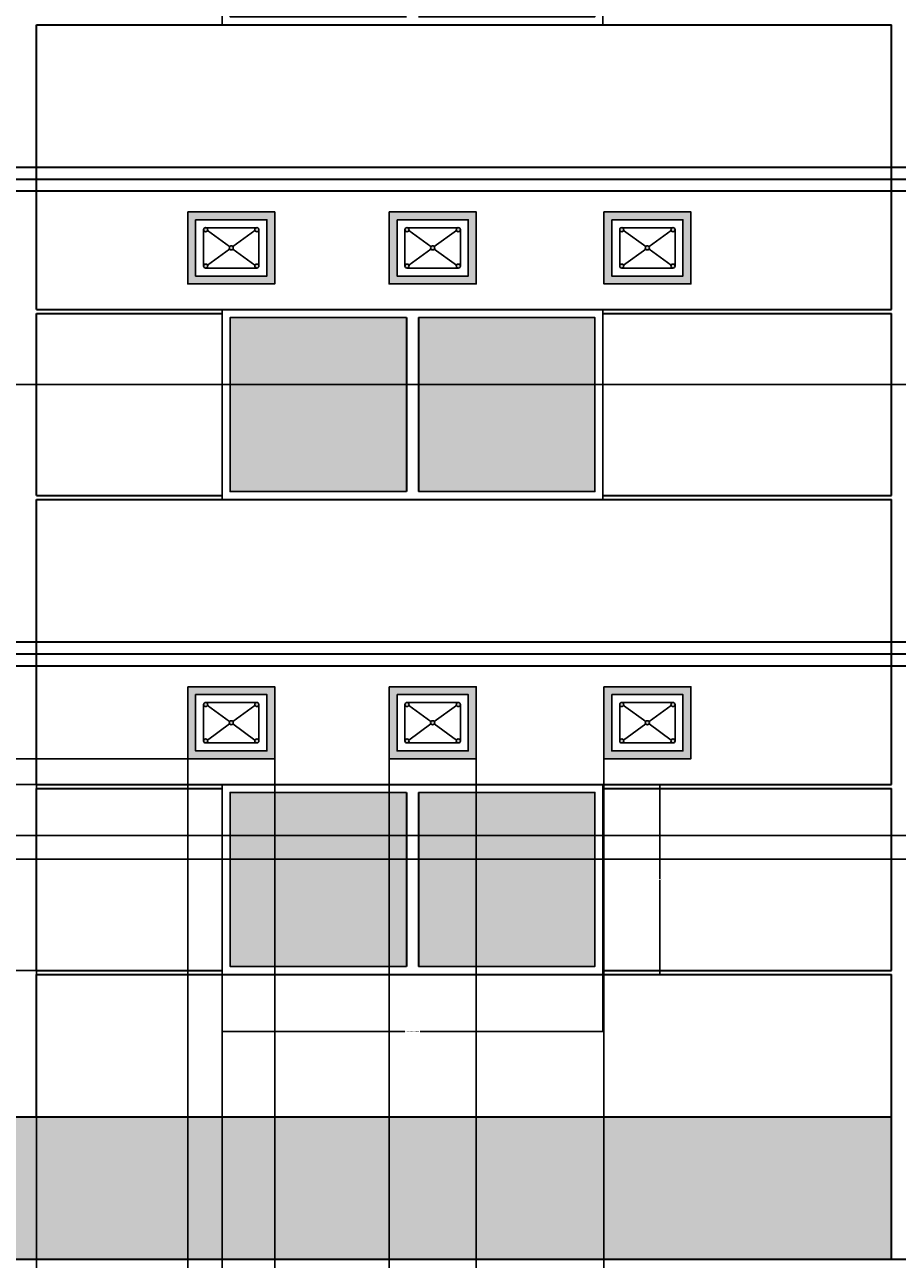
# Model space of a CAD drawing. Units: inches. Extents: x -742 to 1386, y -64 to 951.
# Tile 4 of 8: x 43 to 264, y 106 to 418. Entities that reach past the tile are written whole.
import ezdxf

# ---------------------------------------------------------------- set-up
doc = ezdxf.new("R2010")
doc.units = ezdxf.units.IN
doc.header["$MEASUREMENT"] = 0
for name, color, linetype, lineweight in [('A-ANNO-DIMS', 2, 'Continuous', 18), ('A-ELEV', 7, 'Continuous', 35), ('A-ELEV-PATT', 252, 'Continuous', 13), ('A-GLAZ', 4, 'Continuous', 25), ('A-WALL-PATT', 8, 'Continuous', 13)]:
    doc.layers.add(name, color=color, linetype=linetype, lineweight=lineweight)
doc.styles.get("Standard").update_dxf_attribs({"font": 'arial.ttf'})
doc.dimstyles.get("Standard").update_dxf_attribs({"dimtxt": 0.18, "dimasz": 0.18, "dimexe": 0.18, "dimexo": 0.0625, "dimgap": 0.09, "dimtad": 0, "dimtih": 1, "dimtoh": 1, "dimdec": 4, "dimzin": 0, "dimdsep": 46, "dimtxsty": 'Standard', "dimcen": 0.09, "dimadec": 0, "dimazin": 0, "dimtfac": 1, "dimtdec": 4, "dimtofl": 0, "dimtmove": 0, "dimatfit": 3, "dimfxl": 1, "dimtolj": 1, "dimtzin": 0, "dimarcsym": 0})

# ---------------------------------------------------------------- blocks, each defined once
blk = doc.blocks.new('VENT-WIN')
h = blk.add_hatch(color=256)
h.dxf.hatch_style = 1
h.paths.add_polyline_path([(11.51, 9.11, 1), (10.47, 9.11, 1)])
h.paths.add_polyline_path([(16.95, 13.71, 1), (17.99, 13.71, 1)])
h.paths.add_polyline_path([(17.99, 4.52, 1), (16.95, 4.52, 1)])
h.paths.add_polyline_path([(5.04, 4.52, 1), (4, 4.52, 1)])
h.paths.add_polyline_path([(4, 13.71, 1), (5.04, 13.71, 1)])
for p, q in [((4.99, 13.5), (10.57, 9.42)), ((11.41, 9.42), (16.99, 13.5)), ((4.99, 4.73), (10.57, 8.81)), ((11.41, 8.81), (16.99, 4.73))]:
    blk.add_line(p, q)
for points in [[(0, 18.22), (21.99, 18.22), (21.99, 0), (0, 0)], [(2, 16.22), (19.99, 16.22), (19.99, 2), (2, 2)]]:
    blk.add_lwpolyline(points, close=True)
for points in [[(4, 4.52), (4, 13.71)], [(4.52, 14.22), (17.47, 14.22)], [(17.99, 13.71), (17.99, 4.52)], [(17.47, 4), (4.52, 4)]]:
    blk.add_lwpolyline(points)
for centre in [(4.52, 13.71), (17.47, 13.71), (10.99, 9.11), (4.52, 4.52), (17.47, 4.52)]:
    blk.add_circle(centre, 0.519)
blk = doc.blocks.new('WIN-1000-2PANE')
blk.add_lwpolyline([(0, 48), (96.2, 48), (96.2, 0), (0, 0)], close=True)
for points in [[(46.6, 2), (2, 2), (2, 46), (46.6, 46)], [(49.6, 46), (94.2, 46), (94.2, 2), (49.6, 2)]]:
    blk.add_lwpolyline(points)
blk = doc.blocks.new('*D8')
at = {"layer": 'A-ANNO-DIMS', "color": 0, "lineweight": -2, "transparency": 16777216}
for p, q in [((93.11, 177.68), (93.11, 163.13)), ((189.31, 177.68), (189.31, 163.13)), ((93.29, 163.31), (139.29, 163.31)), ((189.13, 163.31), (143.13, 163.31))]:
    blk.add_line(p, q, dxfattribs=at)
at = {"layer": 'A-ANNO-DIMS', "color": 0, "transparency": 16777216}
for points in [[(93.29, 163.34), (93.29, 163.28), (93.11, 163.31)], [(189.13, 163.34), (189.13, 163.28), (189.31, 163.31)]]:
    blk.add_solid(points, dxfattribs=at)
at = {"layer": 'Defpoints', "color": 0, "transparency": 16777216}
for p in [(93.11, 177.74), (189.31, 177.74), (189.31, 163.31)]:
    blk.add_point(p, dxfattribs=at)
at = {"layer": 'A-ANNO-DIMS', "color": 0, "transparency": 16777216, "insert": (141.21, 163.31), "char_height": 0.18, "attachment_point": 5}
blk.add_mtext('\\A1;WINDOW 1000 2-PANE 96 TYP.', dxfattribs=at)
blk = doc.blocks.new('*D9')
at = {"layer": 'A-ANNO-DIMS', "color": 0, "lineweight": -2, "transparency": 16777216}
for p, q in [((189.38, 225.74), (203.92, 225.74)), ((203.74, 225.56), (203.74, 201.92)), ((203.74, 177.92), (203.74, 201.56)), ((189.38, 177.74), (203.92, 177.74))]:
    blk.add_line(p, q, dxfattribs=at)
at = {"layer": 'A-ANNO-DIMS', "color": 0, "transparency": 16777216}
for points in [[(203.71, 225.56), (203.77, 225.56), (203.74, 225.74)], [(203.71, 177.92), (203.77, 177.92), (203.74, 177.74)]]:
    blk.add_solid(points, dxfattribs=at)
at = {"layer": 'Defpoints', "color": 0, "transparency": 16777216}
for p in [(189.31, 225.74), (203.74, 225.74), (189.31, 177.74)]:
    blk.add_point(p, dxfattribs=at)
at = {"layer": 'A-ANNO-DIMS', "color": 0, "transparency": 16777216, "insert": (203.74, 201.74), "char_height": 0.18, "attachment_point": 5}
blk.add_mtext('\\A1;48 TYP.', dxfattribs=at)
blk = doc.blocks.new('*D20')
at = {"layer": 'A-ANNO-DIMS', "color": 0, "lineweight": -2, "transparency": 16777216}
for p, q in [((40.23, 141.68), (40.23, -63.58)), ((46.23, 141.68), (46.23, -63.58)), ((40.41, -63.4), (43.08, -63.4)), ((46.05, -63.4), (43.38, -63.4))]:
    blk.add_line(p, q, dxfattribs=at)
at = {"layer": 'A-ANNO-DIMS', "color": 0, "transparency": 16777216}
for points in [[(40.41, -63.37), (40.41, -63.43), (40.23, -63.4)], [(46.05, -63.37), (46.05, -63.43), (46.23, -63.4)]]:
    blk.add_solid(points, dxfattribs=at)
at = {"layer": 'Defpoints', "color": 0, "transparency": 16777216}
for p in [(40.23, 141.74), (46.23, 141.74), (46.23, -63.4)]:
    blk.add_point(p, dxfattribs=at)
at = {"layer": 'A-ANNO-DIMS', "color": 0, "transparency": 16777216, "insert": (43.23, -63.4), "char_height": 0.18, "attachment_point": 5}
blk.add_mtext('\\A1;6', dxfattribs=at)
blk = doc.blocks.new('*D25')
at = {"layer": 'A-ANNO-DIMS', "color": 0, "lineweight": -2, "transparency": 16777216}
for p, q in [((46.23, 178.68), (46.23, -63.58)), ((93.11, 178.68), (93.11, -63.58)), ((46.41, -63.4), (69.27, -63.4)), ((92.93, -63.4), (70.07, -63.4))]:
    blk.add_line(p, q, dxfattribs=at)
at = {"layer": 'A-ANNO-DIMS', "color": 0, "transparency": 16777216}
for points in [[(46.41, -63.37), (46.41, -63.43), (46.23, -63.4)], [(92.93, -63.37), (92.93, -63.43), (93.11, -63.4)]]:
    blk.add_solid(points, dxfattribs=at)
at = {"layer": 'Defpoints', "color": 0, "transparency": 16777216}
for p in [(46.23, 178.74), (93.11, 178.74), (93.11, -63.4)]:
    blk.add_point(p, dxfattribs=at)
at = {"layer": 'A-ANNO-DIMS', "color": 0, "transparency": 16777216, "insert": (69.67, -63.4), "char_height": 0.18, "attachment_point": 5}
blk.add_mtext('\\A1;46.88', dxfattribs=at)
blk = doc.blocks.new('*D26')
at = {"layer": 'A-ANNO-DIMS', "color": 0, "lineweight": -2, "transparency": 16777216}
for p, q in [((84.43, 232.16), (84.43, -63.58)), ((46.23, 225.68), (46.23, -63.58)), ((46.41, -63.4), (65, -63.4)), ((84.25, -63.4), (65.65, -63.4))]:
    blk.add_line(p, q, dxfattribs=at)
at = {"layer": 'A-ANNO-DIMS', "color": 0, "transparency": 16777216}
for points in [[(46.41, -63.37), (46.41, -63.43), (46.23, -63.4)], [(84.25, -63.37), (84.25, -63.43), (84.43, -63.4)]]:
    blk.add_solid(points, dxfattribs=at)
at = {"layer": 'Defpoints', "color": 0, "transparency": 16777216}
for p in [(84.43, 232.23), (46.23, 225.74), (84.43, -63.4)]:
    blk.add_point(p, dxfattribs=at)
at = {"layer": 'A-ANNO-DIMS', "color": 0, "transparency": 16777216, "insert": (65.33, -63.4), "char_height": 0.18, "attachment_point": 5}
blk.add_mtext('\\A1;38.2', dxfattribs=at)
blk = doc.blocks.new('*D27')
at = {"layer": 'A-ANNO-DIMS', "color": 0, "lineweight": -2, "transparency": 16777216}
for p, q in [((106.41, 232.16), (106.41, -63.58)), ((135.32, 232.16), (135.32, -63.58)), ((106.59, -63.4), (120.49, -63.4)), ((135.14, -63.4), (121.25, -63.4))]:
    blk.add_line(p, q, dxfattribs=at)
at = {"layer": 'A-ANNO-DIMS', "color": 0, "transparency": 16777216}
for points in [[(106.59, -63.37), (106.59, -63.43), (106.41, -63.4)], [(135.14, -63.37), (135.14, -63.43), (135.32, -63.4)]]:
    blk.add_solid(points, dxfattribs=at)
at = {"layer": 'Defpoints', "color": 0, "transparency": 16777216}
for p in [(106.41, 232.23), (135.32, 232.23), (135.32, -63.4)]:
    blk.add_point(p, dxfattribs=at)
at = {"layer": 'A-ANNO-DIMS', "color": 0, "transparency": 16777216, "insert": (120.87, -63.4), "char_height": 0.18, "attachment_point": 5}
blk.add_mtext('\\A1;28.91', dxfattribs=at)
blk = doc.blocks.new('*D28')
at = {"layer": 'A-ANNO-DIMS', "color": 0, "lineweight": -2, "transparency": 16777216}
for p, q in [((157.31, 232.16), (157.31, -63.58)), ((189.57, 232.16), (189.57, -63.58)), ((157.49, -63.4), (172.98, -63.4)), ((189.39, -63.4), (173.91, -63.4))]:
    blk.add_line(p, q, dxfattribs=at)
at = {"layer": 'A-ANNO-DIMS', "color": 0, "transparency": 16777216}
for points in [[(157.49, -63.37), (157.49, -63.43), (157.31, -63.4)], [(189.39, -63.37), (189.39, -63.43), (189.57, -63.4)]]:
    blk.add_solid(points, dxfattribs=at)
at = {"layer": 'Defpoints', "color": 0, "transparency": 16777216}
for p in [(157.31, 232.23), (189.57, 232.23), (189.57, -63.4)]:
    blk.add_point(p, dxfattribs=at)
at = {"layer": 'A-ANNO-DIMS', "color": 0, "transparency": 16777216, "insert": (173.44, -63.4), "char_height": 0.18, "attachment_point": 5}
blk.add_mtext('\\A1;32.263', dxfattribs=at)
blk = doc.blocks.new('*D49')
at = {"layer": 'A-ANNO-DIMS', "color": 0, "lineweight": -2, "transparency": 16777216}
for p, q in [((93.05, 178.74), (-741.55, 178.74)), ((-741.37, 178.56), (-741.37, 160.42)), ((-741.37, 141.92), (-741.37, 160.06)), ((46.17, 141.74), (-741.55, 141.74))]:
    blk.add_line(p, q, dxfattribs=at)
at = {"layer": 'A-ANNO-DIMS', "color": 0, "transparency": 16777216}
for points in [[(-741.4, 178.56), (-741.34, 178.56), (-741.37, 178.74)], [(-741.4, 141.92), (-741.34, 141.92), (-741.37, 141.74)]]:
    blk.add_solid(points, dxfattribs=at)
at = {"layer": 'Defpoints', "color": 0, "transparency": 16777216}
for p in [(93.11, 178.74), (-741.37, 141.74), (46.23, 141.74)]:
    blk.add_point(p, dxfattribs=at)
at = {"layer": 'A-ANNO-DIMS', "color": 0, "transparency": 16777216, "insert": (-741.37, 160.24), "char_height": 0.18, "attachment_point": 5}
blk.add_mtext('\\A1;37', dxfattribs=at)
blk = doc.blocks.new('*D50')
at = {"layer": 'A-ANNO-DIMS', "color": 0, "lineweight": -2, "transparency": 16777216}
for p, q in [((84.36, 232.23), (-741.55, 232.23)), ((-741.37, 232.05), (-741.37, 229.16)), ((-741.37, 225.92), (-741.37, 228.8)), ((93.05, 225.74), (-741.55, 225.74))]:
    blk.add_line(p, q, dxfattribs=at)
at = {"layer": 'A-ANNO-DIMS', "color": 0, "transparency": 16777216}
for points in [[(-741.4, 232.05), (-741.34, 232.05), (-741.37, 232.23)], [(-741.4, 225.92), (-741.34, 225.92), (-741.37, 225.74)]]:
    blk.add_solid(points, dxfattribs=at)
at = {"layer": 'Defpoints', "color": 0, "transparency": 16777216}
for p in [(-741.37, 232.23), (84.43, 232.23), (93.11, 225.74)]:
    blk.add_point(p, dxfattribs=at)
at = {"layer": 'A-ANNO-DIMS', "color": 0, "transparency": 16777216, "insert": (-741.37, 228.98), "char_height": 0.18, "attachment_point": 5}
blk.add_mtext('\\A1;6.486', dxfattribs=at)
blk = doc.blocks.new('*D55')
at = {"layer": 'A-ANNO-DIMS', "color": 0, "lineweight": -2, "transparency": 16777216}
for p, q in [((295.5, 326.85), (-741.55, 326.85)), ((-741.37, 326.67), (-741.37, 270.04)), ((-741.37, 213.03), (-741.37, 269.67)), ((295.5, 212.85), (-741.55, 212.85))]:
    blk.add_line(p, q, dxfattribs=at)
at = {"layer": 'A-ANNO-DIMS', "color": 0, "transparency": 16777216}
for points in [[(-741.4, 326.67), (-741.34, 326.67), (-741.37, 326.85)], [(-741.4, 213.03), (-741.34, 213.03), (-741.37, 212.85)]]:
    blk.add_solid(points, dxfattribs=at)
at = {"layer": 'Defpoints', "color": 0, "transparency": 16777216}
for p in [(-741.37, 326.85), (295.56, 326.85), (295.56, 212.85)]:
    blk.add_point(p, dxfattribs=at)
at = {"layer": 'A-ANNO-DIMS', "color": 0, "transparency": 16777216, "insert": (-741.37, 269.85), "char_height": 0.18, "attachment_point": 5}
blk.add_mtext('\\A1;114', dxfattribs=at)
blk = doc.blocks.new('*D56')
at = {"layer": 'A-ANNO-DIMS', "color": 0, "lineweight": -2, "transparency": 16777216}
for p, q in [((268.17, 212.85), (-741.55, 212.85)), ((-741.37, 212.67), (-741.37, 210.04)), ((-741.37, 207.03), (-741.37, 209.67)), ((268.17, 206.85), (-741.55, 206.85))]:
    blk.add_line(p, q, dxfattribs=at)
at = {"layer": 'A-ANNO-DIMS', "color": 0, "transparency": 16777216}
for points in [[(-741.4, 212.67), (-741.34, 212.67), (-741.37, 212.85)], [(-741.4, 207.03), (-741.34, 207.03), (-741.37, 206.85)]]:
    blk.add_solid(points, dxfattribs=at)
at = {"layer": 'Defpoints', "color": 0, "transparency": 16777216}
for p in [(-741.37, 212.85), (268.23, 212.85), (268.23, 206.85)]:
    blk.add_point(p, dxfattribs=at)
at = {"layer": 'A-ANNO-DIMS', "color": 0, "transparency": 16777216, "insert": (-741.37, 209.85), "char_height": 0.18, "attachment_point": 5}
blk.add_mtext('\\A1;6', dxfattribs=at)

msp = doc.modelspace()

# ---------------------------------------------------------------- hatches: boundary and pattern name
at = {"layer": 'A-ELEV-PATT'}
h = msp.add_hatch(color=256, dxfattribs=at)
h.dxf.hatch_style = 1
h.paths.add_polyline_path([(106.4136, 370.4496), (84.4263, 370.4496), (84.4263, 352.2254), (106.4136, 352.2254)])
h.paths.add_polyline_path([(104.4136, 354.2254), (86.4263, 354.2254), (86.4263, 368.4496), (104.4136, 368.4496)], flags=16)
h.paths.add_polyline_path([(157.3109, 370.4496), (135.3236, 370.4496), (135.3236, 352.2254), (157.3109, 352.2254)])
h.paths.add_polyline_path([(155.3109, 368.4496), (155.3109, 354.2254), (137.3236, 354.2254), (137.3236, 368.4496)], flags=16)
h.paths.add_polyline_path([(211.5617, 370.4496), (189.5743, 370.4496), (189.5743, 352.2254), (211.5617, 352.2254)])
h.paths.add_polyline_path([(209.5617, 368.4496), (209.5617, 354.2254), (191.5743, 354.2254), (191.5743, 368.4496)], flags=16)
h = msp.add_hatch(color=256, dxfattribs=at)
h.dxf.hatch_style = 1
h.set_gradient(color1=(0, 255, 255), name='CURVED')
h.paths.add_polyline_path([(139.7128, 343.7399), (95.1117, 343.7399), (95.1117, 299.7399), (139.7128, 299.7399)])
h.paths.add_polyline_path([(187.3139, 343.7399), (142.7128, 343.7399), (142.7128, 299.7399), (187.3139, 299.7399)])
h.paths.add_polyline_path([(501.7423, 343.7399), (457.1413, 343.7399), (457.1413, 299.7399), (501.7423, 299.7399)])
h.paths.add_polyline_path([(549.3434, 343.7399), (504.7423, 343.7399), (504.7423, 299.7399), (549.3434, 299.7399)])
h = msp.add_hatch(color=256, dxfattribs=at)
h.dxf.hatch_style = 1
h.paths.add_polyline_path([(106.4136, 250.4496), (84.4263, 250.4496), (84.4263, 232.2254), (106.4136, 232.2254)])
h.paths.add_polyline_path([(104.4136, 234.2254), (86.4263, 234.2254), (86.4263, 248.4496), (104.4136, 248.4496)], flags=16)
h.paths.add_polyline_path([(157.3109, 250.4496), (135.3236, 250.4496), (135.3236, 232.2254), (157.3109, 232.2254)])
h.paths.add_polyline_path([(155.3109, 248.4496), (155.3109, 234.2254), (137.3236, 234.2254), (137.3236, 248.4496)], flags=16)
h.paths.add_polyline_path([(211.5617, 250.4496), (189.5743, 250.4496), (189.5743, 232.2254), (211.5617, 232.2254)])
h.paths.add_polyline_path([(209.5617, 248.4496), (209.5617, 234.2254), (191.5743, 234.2254), (191.5743, 248.4496)], flags=16)
h = msp.add_hatch(color=256, dxfattribs=at)
h.dxf.hatch_style = 1
h.set_gradient(color1=(0, 255, 255), tint=1, name='CURVED')
h.paths.add_polyline_path([(139.7128, 223.7399), (95.1117, 223.7399), (95.1117, 179.7399), (139.7128, 179.7399)])
h.paths.add_polyline_path([(187.3139, 223.7399), (142.7128, 223.7399), (142.7128, 179.7399), (187.3139, 179.7399)])
h.paths.add_polyline_path([(501.7423, 223.7399), (457.1413, 223.7399), (457.1413, 179.7399), (501.7423, 179.7399)])
h.paths.add_polyline_path([(549.3434, 223.7399), (504.7423, 223.7399), (504.7423, 179.7399), (549.3434, 179.7399)])
at = {"layer": 'A-WALL-PATT', "transparency": 33554457}
h = msp.add_hatch(dxfattribs=at)
h.set_pattern_fill('GRAVEL', color=256, scale=40)
h.paths.add_polyline_path([(262.2276, 141.7399), (-37.7724, 141.7399), (-37.7724, 105.7399), (262.2276, 105.7399)])
h.paths.add_polyline_path([(682.2276, 141.7399), (382.2276, 141.7399), (382.2276, 105.7399), (682.2276, 105.7399)])

# ---------------------------------------------------------------- linework, layer by layer
at = {"layer": 'A-ELEV'}
for p, q in [((46.2276, 417.7399), (262.2276, 417.7399)), ((46.2276, 345.7399), (46.2276, 417.7399)), ((262.2276, 345.7399), (262.2276, 417.7399)), ((-37.7724, 381.7399), (268.2276, 381.7399)), ((-37.7724, 378.7399), (268.2276, 378.7399)), ((-37.7724, 375.7399), (268.2276, 375.7399)), ((46.2276, 345.7399), (262.2276, 345.7399)), ((46.2276, 344.7399), (93.1117, 344.7399)), ((46.2276, 298.7399), (46.2276, 344.7399)), ((139.7128, 343.7399), (139.7128, 299.7399)), ((142.7128, 343.7399), (142.7128, 299.7399)), ((189.3139, 344.7399), (262.2276, 344.7399)), ((262.2276, 298.7399), (262.2276, 344.7399)), ((46.2276, 298.7399), (93.1117, 298.7399)), ((46.2276, 225.7399), (46.2276, 297.7399)), ((46.2276, 297.7399), (262.2276, 297.7399)), ((189.3139, 298.7399), (262.2276, 298.7399)), ((262.2276, 225.7399), (262.2276, 297.7399)), ((-37.7724, 261.7399), (268.2276, 261.7399)), ((-37.7724, 258.7399), (268.2276, 258.7399)), ((-37.7724, 255.7399), (268.2276, 255.7399)), ((46.2276, 225.7399), (262.2276, 225.7399)), ((46.2276, 224.7399), (93.1117, 224.7399)), ((46.2276, 178.7399), (46.2276, 224.7399)), ((189.3139, 224.7399), (262.2276, 224.7399)), ((262.2276, 178.7399), (262.2276, 224.7399)), ((139.7128, 223.7399), (139.7128, 179.7399)), ((142.7128, 223.7399), (142.7128, 179.7399)), ((46.2276, 178.7399), (93.1117, 178.7399)), ((189.3139, 178.7399), (262.2276, 178.7399)), ((46.2276, 141.7399), (46.2276, 177.7399)), ((46.2276, 177.7399), (262.2276, 177.7399)), ((262.2276, 105.7399), (262.2276, 177.7399)), ((-37.7724, 141.7399), (262.2276, 141.7399)), ((-37.7724, 105.7399), (262.2276, 105.7399)), ((262.2276, 105.7399), (682.2276, 105.7399))]:
    msp.add_line(p, q, dxfattribs=at)

# ---------------------------------------------------------------- block references
at = {"layer": 'A-GLAZ'}
for name, p in [('WIN-1000-2PANE', (93.112, 417.74)), ('VENT-WIN', (84.4267, 352.225)), ('VENT-WIN', (135.324, 352.225)), ('VENT-WIN', (189.5748, 352.225)), ('WIN-1000-2PANE', (93.112, 297.74)), ('VENT-WIN', (84.4267, 232.225)), ('VENT-WIN', (135.324, 232.225)), ('VENT-WIN', (189.5748, 232.225)), ('WIN-1000-2PANE', (93.112, 177.74))]:
    msp.add_blockref(name, p, dxfattribs=at)

# ---------------------------------------------------------------- dimensions: what is measured, and where the dimension line sits
at = {"layer": 'A-ANNO-DIMS'}
for base, p1, p2, override, picture, middle in [((-741.3711, 326.8548), (295.5643, 212.8548), (295.5643, 326.8548), {"dimdec": 0, "dimlfac": 1, "dimrnd": 0, "dimzin": 0, "dimdsep": 46, "dimlunit": 2}, '*D55', (-741.3711, 269.8548)), ((-741.37107, 232.22544), (93.11175, 225.73986), (84.42625, 232.22544), {"dimdec": 3, "dimlfac": 1, "dimrnd": 0, "dimzin": 0, "dimdsep": 46, "dimlunit": 2}, '*D50', (-741.37107, 228.98265)), ((-741.3711, 212.8548), (268.2276, 206.8548), (268.2276, 212.8548), {"dimdec": 0, "dimlfac": 1, "dimrnd": 0, "dimzin": 0, "dimdsep": 46, "dimlunit": 2}, '*D56', (-741.3711, 209.8548)), ((-741.3711, 141.7399), (93.1117, 178.7399), (46.2276, 141.7399), {"dimdec": 0, "dimlfac": 1, "dimrnd": 0, "dimzin": 0, "dimdsep": 46, "dimlunit": 2}, '*D49', (-741.3711, 160.2399))]:
    dim = msp.add_linear_dim(base=base, p1=p1, p2=p2, angle=90, dimstyle='Standard', override=override, dxfattribs=at)
    dim.commit()
    dim.dimension.update_dxf_attribs({"geometry": picture, "text_midpoint": middle})
for base, p1, p2, override, picture, middle in [((84.4263, -63.3971), (46.2276, 225.7399), (84.4263, 232.2254), {"dimdec": 1, "dimlfac": 1, "dimrnd": 0, "dimzin": 0, "dimdsep": 46, "dimlunit": 2}, '*D26', (65.3269, -63.3971)), ((135.3236, -63.3971), (106.4136, 232.2254), (135.3236, 232.2254), {"dimdec": 2, "dimlfac": 1, "dimrnd": 0, "dimzin": 0, "dimdsep": 46, "dimlunit": 2}, '*D27', (120.8686, -63.3971)), ((189.5743, -63.3971), (157.3109, 232.2254), (189.5743, 232.2254), {"dimdec": 3, "dimlfac": 1, "dimrnd": 0, "dimzin": 0, "dimdsep": 46, "dimlunit": 2}, '*D28', (173.4426, -63.3971)), ((93.1117, -63.3971), (46.2276, 178.7399), (93.1117, 178.7399), {"dimdec": 2, "dimlfac": 1, "dimrnd": 0, "dimzin": 0, "dimdsep": 46, "dimlunit": 2}, '*D25', (69.6697, -63.3971)), ((46.2276, -63.3971), (40.2276, 141.7399), (46.2276, 141.7399), {"dimdec": 0, "dimlfac": 1, "dimrnd": 0, "dimzin": 0, "dimdsep": 46, "dimlunit": 2}, '*D20', (43.2276, -63.3971))]:
    dim = msp.add_linear_dim(base=base, p1=p1, p2=p2, dimstyle='Standard', override=override, dxfattribs=at)
    dim.commit()
    dim.dimension.update_dxf_attribs({"geometry": picture, "text_midpoint": middle})
dim = msp.add_linear_dim(base=(203.7442, 225.7399), p1=(189.3139, 177.7399), p2=(189.3139, 225.7399), angle=90, text='<> TYP.', dimstyle='Standard', override={"dimdec": 0, "dimrnd": 0, "dimzin": 0, "dimlunit": 2}, dxfattribs=at)
dim.commit()
dim.dimension.update_dxf_attribs({"geometry": '*D9', "text_midpoint": (203.7442, 201.7399)})
dim = msp.add_linear_dim(base=(189.3139, 163.3095), p1=(93.1117, 177.7399), p2=(189.3139, 177.7399), text='WINDOW 1000 2-PANE <> TYP.', dimstyle='Standard', override={"dimdec": 0, "dimrnd": 0, "dimzin": 0, "dimlunit": 2}, dxfattribs=at)
dim.commit()
dim.dimension.update_dxf_attribs({"geometry": '*D8', "text_midpoint": (141.2128, 163.3095)})

doc.saveas('drawing.dxf')
